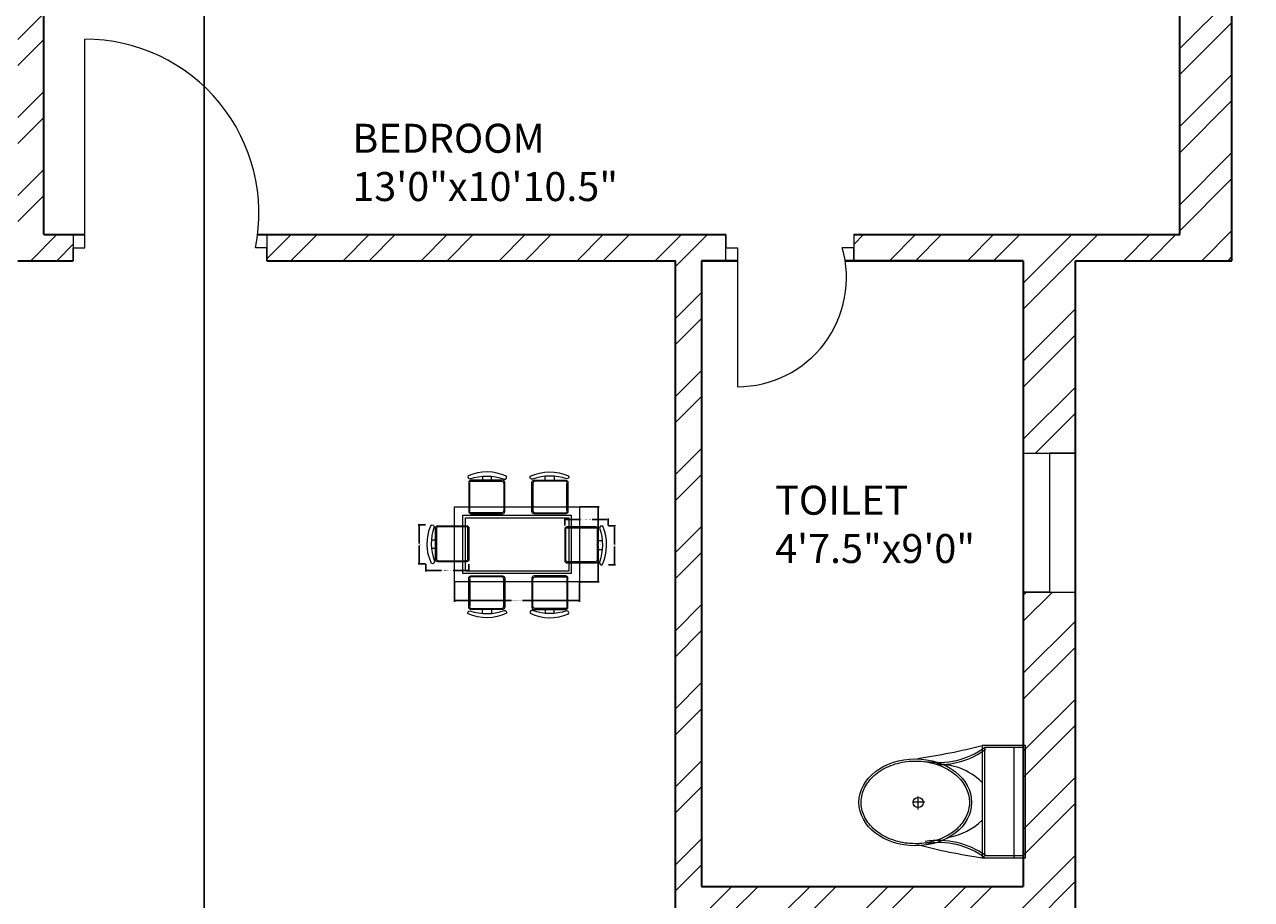
# Model space of a CAD drawing. Units: inches. Extents: x 1513 to 2170, y 1240 to 2288.
# Tile 4 of 10: x 1834 to 2045, y 1549 to 1700. Entities that reach past the tile are written whole.
import ezdxf

# ---------------------------------------------------------------- set-up
doc = ezdxf.new("R2010")
doc.units = ezdxf.units.IN
for name, color, linetype, lineweight in [('A-ANNO-DIMS', 2, 'Continuous', 18), ('A-AREA-IDEN', 7, 'Continuous', 18), ('A-DOOR', 3, 'Continuous', 18), ('A-FLOR-FIXT', 9, 'Continuous', 18), ('A-FURN', 8, 'Continuous', 18), ('A-GLAZ', 4, 'Continuous', 18), ('A-WALL', 7, 'Continuous', 35), ('A-WALL-PATT', 252, 'Continuous', 13)]:
    doc.layers.add(name, color=color, linetype=linetype, lineweight=lineweight)
doc.styles.get("Standard").update_dxf_attribs({"font": 'arial.ttf'})
doc.dimstyles.get("Standard").update_dxf_attribs({"dimtxt": 0.18, "dimasz": 0.18, "dimexe": 0.18, "dimexo": 0.0625, "dimgap": 0.09, "dimtad": 0, "dimtih": 1, "dimtoh": 1, "dimdec": 4, "dimzin": 0, "dimdsep": 46, "dimtxsty": 'Standard', "dimcen": 0.09, "dimadec": 0, "dimazin": 0, "dimtfac": 1, "dimtdec": 4, "dimtofl": 0, "dimtmove": 0, "dimatfit": 3, "dimfxl": 1, "dimtolj": 1, "dimtzin": 0, "dimarcsym": 0})

# ---------------------------------------------------------------- blocks, each defined once
blk = doc.blocks.new('A$C31115884')
for p, q in [((257.5, 466.4), (257.5, 523.2)), ((283.1, 497.7), (223.4, 497.7)), ((0, 200), (0, 0)), ((520, 200), (0, 200)), ((10, 190), (10, 10)), ((510, 190), (10, 190)), ((510, 10), (510, 190)), ((520, 0), (520, 200)), ((510, 54.5), (0, 54.5)), ((10, 10), (510, 10)), ((0, 0), (520, 0))]:
    blk.add_line(p, q)
blk.add_circle((255.6, 496.4), 23.6)
for centre, radius, start, end in [((2777.7, -204.6), 2807, 165.4549, 171.7133), ((-294.5, 403.3), 364.7, 324.2091, 9.3499), ((-294.5, 403.3), 374.7, 324.2091, 9.3499), ((805.8, 403.3), 364.7, 170.6501, 215.7909), ((3237, 905), 2807, 188.2867, 194.5451), ((139.5, 406.2), 293.5, 315.8436, 2.6563), ((805.8, 403.3), 374.7, 179.2036, 215.7909), ((383.6, 406.2), 293.5, 190.2774, 224.1564)]:
    blk.add_arc(centre, radius, start, end)
blk.add_ellipse((256.2, 509.9), major_axis=(0, -260.7), ratio=0.772727)
blk.add_open_spline([(256.2, 259.2), (263.1, 259.2), (270, 259.7), (287.8, 262.3), (298.7, 265.1), (319.9, 273.1), (330.2, 278.4), (350.1, 291.1), (359.7, 298.7), (377.7, 315.9), (386.2, 325.5), (401.7, 346.6), (408.8, 358.1), (421.3, 382.5), (426.8, 395.5), (435.9, 422.4), (439.5, 436.4), (444.8, 465.1), (446.5, 479.7), (447.9, 509.2), (447.6, 524), (445, 553.3), (442.7, 567.8), (436.3, 596), (432.1, 609.7), (421.9, 636), (416, 648.6), (402.5, 672.1), (395, 683), (378.6, 703), (369.8, 712.1), (351.1, 728), (341.3, 734.8), (320.9, 746.2), (310.4, 750.7), (288.9, 757.3), (278, 759.4), (256, 761), (245, 760.6), (223.1, 757.2), (212.3, 754.3), (191.1, 746.1), (180.8, 740.7), (160.9, 727.8), (151.4, 720.1), (133.5, 702.7), (125.1, 693), (109.6, 671.7), (102.6, 660.2), (90.2, 635.7), (84.9, 622.7), (76, 595.6), (72.4, 581.6), (67.2, 552.9), (65.6, 538.2), (64.4, 508.8), (64.8, 494), (67.5, 464.7), (69.9, 450.2), (76.6, 422), (80.8, 408.3), (91.1, 382.2), (97.2, 369.7), (110.8, 346.3), (118.4, 335.4), (134.8, 315.6), (143.7, 306.7), (162.4, 290.9), (172.3, 284.2), (192.8, 273), (203.3, 268.6), (224.8, 262.2), (235.8, 260.2), (249.9, 259.3), (253, 259.2), (256.2, 259.2)], degree=3, knots=[0, 0, 0, 0, 0.110105, 0.110105, 0.285049, 0.285049, 0.459994, 0.459994, 0.634938, 0.634938, 0.809882, 0.809882, 0.984827, 0.984827, 1.159771, 1.159771, 1.334715, 1.334715, 1.50966, 1.50966, 1.684604, 1.684604, 1.859549, 1.859549, 2.034493, 2.034493, 2.209437, 2.209437, 2.384382, 2.384382, 2.559326, 2.559326, 2.73427, 2.73427, 2.909215, 2.909215, 3.084159, 3.084159, 3.259103, 3.259103, 3.434048, 3.434048, 3.608992, 3.608992, 3.783936, 3.783936, 3.958881, 3.958881, 4.133825, 4.133825, 4.30877, 4.30877, 4.483714, 4.483714, 4.658658, 4.658658, 4.833603, 4.833603, 5.008547, 5.008547, 5.183491, 5.183491, 5.358436, 5.358436, 5.53338, 5.53338, 5.708324, 5.708324, 5.883269, 5.883269, 6.058213, 6.058213, 6.233158, 6.233158, 6.283185, 6.283185, 6.283185, 6.283185])
blk = doc.blocks.new('WIN-24')
for p, q in [((0, 24), (9, 24)), ((9, 24), (4.5, 24)), ((4.5, 24), (4.5, 0)), ((4.5, 0), (0, 0)), ((0, 0), (9, 0))]:
    blk.add_line(p, q)
blk = doc.blocks.new('TABLE-DINING')
for points in [[(0, 12.94), (21.57, 12.94), (21.57, 0), (0, 0)], [(0, 12.94), (21.57, 12.94), (21.57, 0), (0, 0)], [(1.44, 11.51), (20.13, 11.51), (20.13, 1.44), (1.44, 1.44)], [(1.44, 11.5), (20.13, 11.5), (20.13, 1.44), (1.44, 1.44)], [(1.87, 11.07), (19.7, 11.07), (19.7, 1.87), (1.87, 1.87)], [(1.87, 11.07), (19.7, 11.07), (19.7, 1.87), (1.87, 1.87)]]:
    blk.add_lwpolyline(points, close=True)
blk = doc.blocks.new('CHAIR-DINING-A')
for points in [[(0.35, 6.01, -0.175809), (6.23, 5.97, 0.578392), (6.67, 6.46, 0.214524), (0.04, 6.55, 0.552014), (0.35, 6.01, -0.065079)], [(0.35, 6.01, -0.175809), (6.23, 5.97, 0.578392), (6.67, 6.46, 0.214524), (0.04, 6.55, 0.552014), (0.35, 6.01, -0.065079)], [(4.06, 5.78), (4.06, 6.47, -0.064759)], [(4.06, 5.78), (4.06, 6.47, -0.064759)], [(5.98, 5.78), (0.53, 5.78, 0.414214), (0.14, 5.4), (0.14, 0.38, 0.414214), (0.53, 0), (5.98, 0, 0.414214), (6.36, 0.38), (6.36, 5.4, 0.414214), (5.98, 5.78)], [(5.98, 5.78), (0.53, 5.78, 0.414214), (0.14, 5.4), (0.14, 0.38, 0.414214), (0.53, 0), (5.98, 0, 0.414214), (6.36, 0.38), (6.36, 5.4, 0.414214), (5.98, 5.78)]]:
    blk.add_lwpolyline(points, format="xyb")
blk.add_lwpolyline([(2.54, 6.48), (2.54, 5.78)])
blk.add_lwpolyline([(2.54, 6.48), (2.54, 5.78)])
blk.add_lwpolyline([(0.53, 5.61), (5.81, 5.61, -0.414214), (6.19, 5.23), (6.19, 0.55, -0.414214), (5.81, 0.17), (0.53, 0.17, -0.512069), (0.32, 0.55), (0.32, 5.23, -0.512069)], format="xyb", close=True)
blk.add_lwpolyline([(0.53, 5.61), (5.81, 5.61, -0.414214), (6.19, 5.23), (6.19, 0.55, -0.414214), (5.81, 0.17), (0.53, 0.17, -0.512069), (0.32, 0.55), (0.32, 5.23, -0.512069)], format="xyb", close=True)
blk = doc.blocks.new('CHAIR-DINING-B')
for points in [[(5.98, 1.44), (0.53, 1.44, -0.414214), (0.14, 1.82), (0.14, 6.83, -0.414214), (0.53, 7.22), (5.98, 7.22, -0.414214), (6.36, 6.83), (6.36, 1.82, -0.414214), (5.98, 1.44)], [(5.98, 1.44), (0.53, 1.44, -0.414214), (0.14, 1.82), (0.14, 6.83, -0.414214), (0.53, 7.22), (5.98, 7.22, -0.414214), (6.36, 6.83), (6.36, 1.82, -0.414214), (5.98, 1.44)], [(6.23, 1.25, -0.578392), (6.67, 0.76, -0.214524), (0.04, 0.67, -0.552014), (0.35, 1.2, 0.175809), (6.23, 1.25)], [(6.23, 1.25, -0.578392), (6.67, 0.76, -0.214524), (0.04, 0.67, -0.552014), (0.35, 1.2, 0.175809), (6.23, 1.25)], [(4.06, 1.44), (4.06, 0.75, 0.064759)], [(4.06, 1.44), (4.06, 0.75, 0.064759)]]:
    blk.add_lwpolyline(points, format="xyb")
blk.add_lwpolyline([(0.53, 1.61), (5.81, 1.61, 0.414214), (6.19, 1.99), (6.19, 6.66, 0.414214), (5.81, 7.04), (0.53, 7.04, 0.512069), (0.32, 6.66), (0.32, 1.99, 0.512069)], format="xyb", close=True)
blk.add_lwpolyline([(0.53, 1.61), (5.81, 1.61, 0.414214), (6.19, 1.99), (6.19, 6.66, 0.414214), (5.81, 7.04), (0.53, 7.04, 0.512069), (0.32, 6.66), (0.32, 1.99, 0.512069)], format="xyb", close=True)
blk.add_lwpolyline([(2.54, 0.74), (2.54, 1.44)])
blk.add_lwpolyline([(2.54, 0.74), (2.54, 1.44)])
blk = doc.blocks.new('*D17')
at = {"layer": 'A-ANNO-DIMS', "color": 0, "lineweight": -2, "transparency": 16777216}
for p, q in [((1926.73, 1613.76), (1926.73, 1615)), ((1926.91, 1614.82), (1929.47, 1614.82)), ((1934.02, 1614.82), (1931.47, 1614.82)), ((1934.2, 1613.76), (1934.2, 1615))]:
    blk.add_line(p, q, dxfattribs=at)
at = {"layer": 'A-ANNO-DIMS', "color": 0, "transparency": 16777216}
for points in [[(1926.91, 1614.85), (1926.91, 1614.79), (1926.73, 1614.82)], [(1934.02, 1614.85), (1934.02, 1614.79), (1934.2, 1614.82)]]:
    blk.add_solid(points, dxfattribs=at)
at = {"layer": 'Defpoints', "color": 0, "transparency": 16777216}
for p in [(1926.73, 1613.7), (1934.2, 1614.82), (1934.2, 1613.7)]:
    blk.add_point(p, dxfattribs=at)
at = {"layer": 'A-ANNO-DIMS', "color": 0, "transparency": 16777216, "insert": (1930.47, 1614.82), "char_height": 0.18, "attachment_point": 5}
blk.add_mtext('\\A1;CHAIR A 7 TYP.', dxfattribs=at)
blk = doc.blocks.new('*D18')
at = {"layer": 'A-ANNO-DIMS', "color": 0, "lineweight": -2, "transparency": 16777216}
for p, q in [((1934.26, 1613.7), (1935.5, 1613.7)), ((1935.32, 1613.52), (1935.32, 1610.51)), ((1935.32, 1607.15), (1935.32, 1610.15)), ((1934.26, 1606.97), (1935.5, 1606.97))]:
    blk.add_line(p, q, dxfattribs=at)
at = {"layer": 'A-ANNO-DIMS', "color": 0, "transparency": 16777216}
for points in [[(1935.29, 1613.52), (1935.35, 1613.52), (1935.32, 1613.7)], [(1935.29, 1607.15), (1935.35, 1607.15), (1935.32, 1606.97)]]:
    blk.add_solid(points, dxfattribs=at)
at = {"layer": 'Defpoints', "color": 0, "transparency": 16777216}
for p in [(1934.2, 1613.7), (1934.2, 1606.97), (1935.32, 1606.97)]:
    blk.add_point(p, dxfattribs=at)
at = {"layer": 'A-ANNO-DIMS', "color": 0, "transparency": 16777216, "insert": (1935.32, 1610.33), "char_height": 0.18, "attachment_point": 5}
blk.add_mtext('\\A1;7 TYP.', dxfattribs=at)
blk = doc.blocks.new('*D19')
at = {"layer": 'A-ANNO-DIMS', "color": 0, "lineweight": -2, "transparency": 16777216}
for p, q in [((1902.74, 1607.09), (1902.74, 1605.85)), ((1910.21, 1607.09), (1910.21, 1605.85)), ((1902.92, 1606.03), (1905.47, 1606.03)), ((1910.03, 1606.03), (1907.47, 1606.03))]:
    blk.add_line(p, q, dxfattribs=at)
at = {"layer": 'A-ANNO-DIMS', "color": 0, "transparency": 16777216}
for points in [[(1902.92, 1606.06), (1902.92, 1606), (1902.74, 1606.03)], [(1910.03, 1606.06), (1910.03, 1606), (1910.21, 1606.03)]]:
    blk.add_solid(points, dxfattribs=at)
at = {"layer": 'Defpoints', "color": 0, "transparency": 16777216}
for p in [(1902.74, 1607.15), (1910.21, 1607.15), (1910.21, 1606.03)]:
    blk.add_point(p, dxfattribs=at)
at = {"layer": 'A-ANNO-DIMS', "color": 0, "transparency": 16777216, "insert": (1906.47, 1606.03), "char_height": 0.18, "attachment_point": 5}
blk.add_mtext('\\A1;CHAIR B 7 TYP.', dxfattribs=at)
blk = doc.blocks.new('*D20')
at = {"layer": 'A-ANNO-DIMS', "color": 0, "lineweight": -2, "transparency": 16777216}
for p, q in [((1902.68, 1613.89), (1901.44, 1613.89)), ((1901.62, 1613.71), (1901.62, 1610.7)), ((1901.62, 1607.33), (1901.62, 1610.34)), ((1902.68, 1607.15), (1901.44, 1607.15))]:
    blk.add_line(p, q, dxfattribs=at)
at = {"layer": 'A-ANNO-DIMS', "color": 0, "transparency": 16777216}
for points in [[(1901.59, 1613.71), (1901.65, 1613.71), (1901.62, 1613.89)], [(1901.59, 1607.33), (1901.65, 1607.33), (1901.62, 1607.15)]]:
    blk.add_solid(points, dxfattribs=at)
at = {"layer": 'Defpoints', "color": 0, "transparency": 16777216}
for p in [(1902.74, 1613.89), (1901.62, 1607.15), (1902.74, 1607.15)]:
    blk.add_point(p, dxfattribs=at)
at = {"layer": 'A-ANNO-DIMS', "color": 0, "transparency": 16777216, "insert": (1901.62, 1610.52), "char_height": 0.18, "attachment_point": 5}
blk.add_mtext('\\A1;7 TYP.', dxfattribs=at)
blk = doc.blocks.new('*D21')
at = {"layer": 'A-ANNO-DIMS', "color": 0, "lineweight": -2, "transparency": 16777216}
for p, q in [((1907.71, 1603.98), (1907.71, 1600.63)), ((1929.28, 1603.98), (1929.28, 1600.63)), ((1907.89, 1600.81), (1917.53, 1600.81)), ((1929.1, 1600.81), (1919.46, 1600.81))]:
    blk.add_line(p, q, dxfattribs=at)
at = {"layer": 'A-ANNO-DIMS', "color": 0, "transparency": 16777216}
for points in [[(1907.89, 1600.84), (1907.89, 1600.78), (1907.71, 1600.81)], [(1929.1, 1600.84), (1929.1, 1600.78), (1929.28, 1600.81)]]:
    blk.add_solid(points, dxfattribs=at)
at = {"layer": 'Defpoints', "color": 0, "transparency": 16777216}
for p in [(1907.71, 1604.04), (1929.28, 1604.04), (1929.28, 1600.81)]:
    blk.add_point(p, dxfattribs=at)
at = {"layer": 'A-ANNO-DIMS', "color": 0, "transparency": 16777216, "insert": (1918.5, 1600.81), "char_height": 0.18, "attachment_point": 5}
blk.add_mtext('\\A1;TABLE 22 TYP.', dxfattribs=at)
blk = doc.blocks.new('*D22')
at = {"layer": 'A-ANNO-DIMS', "color": 0, "lineweight": -2, "transparency": 16777216}
for p, q in [((1929.35, 1616.99), (1932.7, 1616.99)), ((1932.52, 1616.81), (1932.52, 1610.7)), ((1932.52, 1604.22), (1932.52, 1610.33)), ((1929.35, 1604.04), (1932.7, 1604.04))]:
    blk.add_line(p, q, dxfattribs=at)
at = {"layer": 'A-ANNO-DIMS', "color": 0, "transparency": 16777216}
for points in [[(1932.49, 1616.81), (1932.55, 1616.81), (1932.52, 1616.99)], [(1932.49, 1604.22), (1932.55, 1604.22), (1932.52, 1604.04)]]:
    blk.add_solid(points, dxfattribs=at)
at = {"layer": 'Defpoints', "color": 0, "transparency": 16777216}
for p in [(1929.28, 1616.99), (1932.52, 1616.99), (1929.28, 1604.04)]:
    blk.add_point(p, dxfattribs=at)
at = {"layer": 'A-ANNO-DIMS', "color": 0, "transparency": 16777216, "insert": (1932.52, 1610.52), "char_height": 0.18, "attachment_point": 5}
blk.add_mtext('\\A1;13 TYP.', dxfattribs=at)
blk = doc.blocks.new('*D26')
at = {"layer": 'A-ANNO-DIMS', "color": 0, "lineweight": -2, "transparency": 16777216}
for p, q in [((2014.91, 2214.48), (2087.18, 2214.48)), ((2087, 2214.3), (2087, 1802.16)), ((2087, 1389.66), (2087, 1801.8)), ((1937.43, 1389.48), (2087.18, 1389.48))]:
    blk.add_line(p, q, dxfattribs=at)
at = {"layer": 'A-ANNO-DIMS', "color": 0, "transparency": 16777216}
for points in [[(2086.97, 2214.3), (2087.03, 2214.3), (2087, 2214.48)], [(2086.97, 1389.66), (2087.03, 1389.66), (2087, 1389.48)]]:
    blk.add_solid(points, dxfattribs=at)
at = {"layer": 'Defpoints', "color": 0, "transparency": 16777216}
for p in [(2014.85, 2214.48), (2087, 2214.48), (1937.37, 1389.48)]:
    blk.add_point(p, dxfattribs=at)
at = {"layer": 'A-ANNO-DIMS', "color": 0, "transparency": 16777216, "insert": (2087, 1801.98), "char_height": 0.18, "attachment_point": 5}
blk.add_mtext('\\A1;825', dxfattribs=at)
blk = doc.blocks.new('*D36')
at = {"layer": 'A-ANNO-DIMS', "color": 0, "lineweight": -2, "transparency": 16777216}
for p, q in [((1829.49, 1887.42), (1829.49, 1344.15)), ((1864.51, 1887.42), (1864.51, 1344.15)), ((1829.67, 1344.33), (1846.61, 1344.33)), ((1864.33, 1344.33), (1847.39, 1344.33))]:
    blk.add_line(p, q, dxfattribs=at)
at = {"layer": 'A-ANNO-DIMS', "color": 0, "transparency": 16777216}
for points in [[(1829.67, 1344.36), (1829.67, 1344.3), (1829.49, 1344.33)], [(1864.33, 1344.36), (1864.33, 1344.3), (1864.51, 1344.33)]]:
    blk.add_solid(points, dxfattribs=at)
at = {"layer": 'Defpoints', "color": 0, "transparency": 16777216}
for p in [(1829.49, 1887.48), (1864.51, 1887.48), (1864.51, 1344.33)]:
    blk.add_point(p, dxfattribs=at)
at = {"layer": 'A-ANNO-DIMS', "color": 0, "transparency": 16777216, "insert": (1847, 1344.33), "char_height": 0.18, "attachment_point": 5}
blk.add_mtext('\\A1;35.02', dxfattribs=at)

msp = doc.modelspace()

# ---------------------------------------------------------------- hatches: boundary and pattern name
at = {"layer": 'A-WALL-PATT'}
h = msp.add_hatch(dxfattribs=at)
h.set_pattern_fill('ANSI32', color=256)
h.paths.add_polyline_path([(2041.852, 1719.48), (2014.852, 1719.48), (2014.852, 1734.444), (2005.852, 1734.444), (2005.852, 1710.48), (2032.852, 1710.48), (2032.852, 1663.98), (1976.619, 1663.98), (1976.619, 1659.48), (2005.852, 1659.48), (2005.852, 1626.27), (2014.852, 1626.27), (2014.852, 1659.48), (2041.852, 1659.48)])
h.paths.add_polyline_path([(1954.521, 1663.98), (1875.357, 1663.98), (1875.357, 1659.48), (1945.852, 1659.48), (1945.852, 1546.98), (1950.352, 1546.98), (2005.852, 1546.98), (2005.852, 1422.48), (1985.47, 1422.48), (1985.47, 1413.48), (2014.852, 1413.48), (2014.852, 1602.27), (2005.852, 1602.27), (2005.852, 1551.48), (1950.352, 1551.48), (1950.352, 1659.48), (1954.521, 1659.48)])
h.paths.add_polyline_path([(1949.47, 1422.48), (1937.366, 1422.48), (1937.366, 1413.48), (1949.47, 1413.48)], flags=0)
h.paths.add_polyline_path([(1937.366, 1422.48), (1908.866, 1422.48), (1908.866, 1546.98), (1805.486, 1546.98), (1805.486, 1542.48), (1904.366, 1542.48), (1904.366, 1451.2), (1897.222, 1451.2), (1897.222, 1442.2), (1904.366, 1442.2), (1904.366, 1422.48), (1904.366, 1413.48), (1904.366, 1389.48), (1908.866, 1389.48), (1908.866, 1413.48), (1932.866, 1413.48), (1932.866, 1389.48), (1937.366, 1389.48)])
h.paths.add_polyline_path([(1830.254, 1442.2), (1844.144, 1442.2), (1844.144, 1451.2), (1830.254, 1451.2), (1821.254, 1451.2), (1821.254, 1422.48), (1766.366, 1422.48), (1766.366, 1542.48), (1770.265, 1542.48), (1770.265, 1546.98), (1758.774, 1546.98), (1758.774, 1544.73), (1758.774, 1542.48), (1761.866, 1542.48), (1761.866, 1389.48), (1779.454, 1389.48), (1779.454, 1398.48), (1770.866, 1398.48), (1770.866, 1413.48), (1830.254, 1413.48)])
h.paths.add_polyline_path([(1686.156, 1451.2), (1677.156, 1451.2), (1677.156, 1422.48), (1623.866, 1422.48), (1623.866, 1460.073), (1614.866, 1460.073), (1614.866, 1413.48), (1686.156, 1413.48)])
h.paths.add_polyline_path([(1761.866, 1422.48), (1686.156, 1422.48), (1686.156, 1413.48), (1761.866, 1413.48)])
h.paths.add_polyline_path([(1623.866, 1542.48), (1688.266, 1542.48), (1688.266, 1544.73), (1688.266, 1546.98), (1623.866, 1546.98), (1623.866, 1560.442), (1614.866, 1560.442), (1614.866, 1520.073), (1619.366, 1520.073), (1623.866, 1520.073)])
h.paths.add_polyline_path([(1623.866, 1600.98), (1715.366, 1600.98), (1715.366, 1546.98), (1711.055, 1546.98), (1711.055, 1542.48), (1719.866, 1542.48), (1726.867, 1542.48), (1726.867, 1544.73), (1726.867, 1546.98), (1719.866, 1546.98), (1719.866, 1600.98), (1719.866, 1608.301), (1717.616, 1608.301), (1715.366, 1608.301), (1715.366, 1605.48), (1623.866, 1605.48), (1623.866, 1620.254), (1614.866, 1620.254), (1614.866, 1584.442), (1623.866, 1584.442)])
h.paths.add_polyline_path([(1623.866, 1659.48), (1715.366, 1659.48), (1715.366, 1629.2), (1719.866, 1629.2), (1719.866, 1659.48), (1767.866, 1659.48), (1767.866, 1629.2), (1772.366, 1629.2), (1772.366, 1663.98), (1578.866, 1663.98), (1578.866, 1661.73), (1578.866, 1659.48), (1578.866, 1635.48), (1583.366, 1635.48), (1583.366, 1654.98), (1614.866, 1654.98), (1614.866, 1644.254), (1619.366, 1644.254), (1623.866, 1644.254)])
h.paths.add_polyline_path([(1788.587, 1798.98), (1788.587, 1803.48), (1623.866, 1803.48), (1623.866, 1887.48), (1829.49, 1887.48), (1829.49, 1891.98), (1829.49, 1896.48), (1748.366, 1896.48), (1743.866, 1896.48), (1623.866, 1896.48), (1623.866, 1904.333), (1619.366, 1904.333), (1614.866, 1904.333), (1614.866, 1896.48), (1578.866, 1896.48), (1578.866, 1887.48), (1614.866, 1887.48), (1614.866, 1803.48), (1578.866, 1803.48), (1578.866, 1794.48), (1626.866, 1794.48), (1788.587, 1794.48)])
h.paths.add_polyline_path([(1635.866, 1794.48), (1626.866, 1794.48), (1626.866, 1763.627), (1631.366, 1763.627), (1635.866, 1763.627)])
h.paths.add_polyline_path([(1635.866, 1703.627), (1626.866, 1703.627), (1626.866, 1663.98), (1635.866, 1663.98)])
h.paths.add_polyline_path([(1587.866, 2016.48), (1614.866, 2016.48), (1623.866, 2016.48), (1707.767, 2016.48), (1707.767, 2018.73), (1707.767, 2020.98), (1706.366, 2020.98), (1706.366, 2025.944), (1701.866, 2025.944), (1701.866, 2020.98), (1623.866, 2020.98), (1623.866, 2045.903), (1614.866, 2045.903), (1614.866, 2025.48), (1583.366, 2025.48), (1583.366, 2040.48), (1578.866, 2040.48), (1578.866, 2016.48), (1578.866, 1956.48), (1614.866, 1956.48), (1614.866, 1946.333), (1623.866, 1946.333), (1623.866, 1965.48), (1587.866, 1965.48)])
h.paths.add_polyline_path([(1748.366, 2016.48), (1748.366, 2025.48), (1743.866, 2025.48), (1739.366, 2025.48), (1739.366, 2020.98), (1738.09, 2020.98), (1738.09, 2016.48), (1743.866, 2016.48), (1743.866, 1896.48), (1748.366, 1896.48)])
h.paths.add_polyline_path([(1746.736, 2085.48), (1623.866, 2085.48), (1623.866, 2205.48), (1657.136, 2205.48), (1657.136, 2214.48), (1614.866, 2214.48), (1614.866, 2069.903), (1623.866, 2069.903), (1623.866, 2080.98), (1683.866, 2080.98), (1701.866, 2080.98), (1701.866, 2046.743), (1706.366, 2046.743), (1706.366, 2080.98), (1746.736, 2080.98)])
h = msp.add_hatch(dxfattribs=at)
h.set_pattern_fill('ANSI32', color=256)
h.paths.add_polyline_path([(1744.852, 2209.98), (1762.042, 2209.98), (1762.042, 2214.48), (1715.345, 2214.48), (1715.345, 2205.48), (1735.852, 2205.48), (1735.852, 2161.98), (1733.253, 2161.98), (1719.866, 2161.98), (1719.866, 2112.429), (1724.366, 2112.429), (1724.366, 2152.98), (1762.042, 2152.98), (1870.852, 2152.98), (1870.852, 2080.98), (1875.352, 2080.98), (1878.245, 2080.98), (1878.245, 2083.23), (1878.245, 2085.48), (1875.352, 2085.48), (1875.352, 2173.929), (1881.628, 2173.929), (1881.628, 2178.429), (1881.628, 2182.929), (1875.352, 2182.929), (1875.352, 2214.48), (1858.335, 2214.48), (1858.335, 2209.98), (1866.352, 2209.98), (1866.352, 2161.98), (1762.042, 2161.98), (1744.852, 2161.98)])
h.paths.add_polyline_path([(2014.852, 2214.48), (1944.011, 2214.48), (1944.011, 2182.929), (1938.347, 2182.929), (1938.347, 2173.929), (1953.011, 2173.929), (1953.011, 2182.929), (1953.011, 2205.48), (2005.852, 2205.48), (2005.852, 2085.48), (1955.061, 2085.48), (1955.061, 2080.98), (2005.852, 2080.98), (2005.852, 2068.903), (2014.852, 2068.903)])
h.paths.add_polyline_path([(2014.852, 2044.903), (2005.852, 2044.903), (2005.852, 2020.98), (1926.352, 2020.98), (1926.352, 2080.98), (1930.882, 2080.98), (1930.882, 2083.23), (1930.882, 2085.48), (1921.852, 2085.48), (1915.536, 2085.48), (1915.536, 2083.23), (1915.536, 2080.98), (1921.852, 2080.98), (1921.852, 2020.98), (1916.378, 2020.98), (1916.378, 2018.73), (1916.378, 2016.48), (2005.852, 2016.48), (2005.852, 2009.442), (2014.852, 2009.442), (2014.852, 2016.48), (2029.852, 2016.48), (2041.852, 2016.48), (2041.852, 2040.48), (2037.352, 2040.48), (2037.352, 2036.595), (2037.352, 2020.98), (2014.852, 2020.98)])
h.paths.add_polyline_path([(2041.852, 1956.48), (2014.852, 1956.48), (2014.852, 1963.797), (2005.852, 1963.797), (2005.852, 1947.48), (2032.852, 1947.48), (2032.852, 1896.48), (1978.852, 1896.48), (1978.852, 1891.98), (1978.852, 1887.48), (2005.852, 1887.48), (2005.852, 1862.401), (2014.852, 1862.401), (2014.852, 1887.48), (2037.352, 1887.48), (2037.352, 1863.48), (2041.852, 1863.48), (2041.852, 1887.48), (2041.852, 1896.48)], flags=17)
h.paths.add_polyline_path([(1885.852, 1896.48), (1885.852, 1920.48), (1878.866, 1920.48), (1878.866, 2016.48), (1881.925, 2016.48), (1881.925, 2018.73), (1881.925, 2020.98), (1874.366, 2020.98), (1874.366, 1896.48), (1864.508, 1896.48), (1864.508, 1887.48), (1876.852, 1887.48), (1876.852, 1855.773), (1885.852, 1855.773), (1885.852, 1868.947), (1942.852, 1868.947), (1942.852, 1803.48), (1885.852, 1803.48), (1885.852, 1817.861), (1876.852, 1817.861), (1876.852, 1803.48), (1825.976, 1803.48), (1825.976, 1798.98), (1825.976, 1794.48), (1832.366, 1794.48), (1832.366, 1663.98), (1832.366, 1659.48), (1841.939, 1659.48), (1841.939, 1661.73), (1841.939, 1663.98), (1836.866, 1663.98), (1836.866, 1794.48), (1992.866, 1794.48), (2005.852, 1794.48), (2005.852, 1784.304), (2010.352, 1784.304), (2014.852, 1784.304), (2014.852, 1794.48), (2041.852, 1794.48), (2041.852, 1803.48), (2014.852, 1803.48), (2014.852, 1838.401), (2005.852, 1838.401), (2005.852, 1803.48), (1951.852, 1803.48), (1951.852, 1887.48), (1956.114, 1887.48), (1956.114, 1891.98), (1956.114, 1896.48), (1951.852, 1896.48), (1951.852, 1920.48), (1947.352, 1920.48), (1947.352, 1896.48), (1942.852, 1896.48), (1942.852, 1877.947), (1885.852, 1877.947)])

# ---------------------------------------------------------------- linework, layer by layer
at = {"layer": 'A-DOOR'}
for p, q in [((1843.939, 1661.73), (1843.939, 1697.73)), ((1841.939, 1663.98), (1841.939, 1659.48)), ((1875.357, 1663.98), (1875.357, 1659.48)), ((1954.521, 1659.48), (1954.521, 1663.98)), ((1954.521, 1663.98), (1954.521, 1661.73)), ((1976.619, 1663.98), (1976.619, 1659.48)), ((1841.939, 1659.48), (1841.939, 1661.73)), ((1841.939, 1661.73), (1843.939, 1661.73)), ((1875.357, 1661.73), (1873.357, 1661.73)), ((1875.357, 1659.48), (1875.357, 1661.73)), ((1954.521, 1661.73), (1956.521, 1661.73)), ((1956.521, 1661.73), (1956.521, 1637.73)), ((1976.619, 1661.73), (1974.619, 1661.73)), ((1976.619, 1659.48), (1976.619, 1661.73))]:
    msp.add_line(p, q, dxfattribs=at)
for centre, radius, start, end in [((1843.939, 1667.71), 30.02, 348.50896, 90), ((1956.521, 1656.553), 18.823, 270, 15.96234)]:
    msp.add_arc(centre, radius, start, end, dxfattribs=at)
at = {"layer": 'A-FURN'}
for points in [[(1910.382, 1621.827, -0.1758092), (1916.257, 1621.783, 0.5783921), (1916.702, 1622.272, 0.2145244), (1910.071, 1622.361, 0.552014), (1910.382, 1621.827, -0.065079)], [(1910.382, 1621.827, -0.1758092), (1916.257, 1621.783, 0.5783921), (1916.702, 1622.272, 0.2145244), (1910.071, 1622.361, 0.552014), (1910.382, 1621.827, -0.065079)], [(1914.092, 1621.592), (1914.092, 1622.281, -0.0647586)], [(1914.092, 1621.591), (1914.092, 1622.281, -0.0647586)], [(1916.007, 1621.592), (1910.554, 1621.592, 0.4142136), (1910.172, 1621.21), (1910.172, 1616.195, 0.4142136), (1910.554, 1615.814), (1916.007, 1615.814, 0.4142136), (1916.389, 1616.195), (1916.389, 1621.21, 0.4142136), (1916.007, 1621.592)], [(1916.007, 1621.591), (1910.554, 1621.591, 0.4142136), (1910.172, 1621.21), (1910.172, 1616.195, 0.4142136), (1910.554, 1615.814), (1916.007, 1615.814, 0.4142136), (1916.389, 1616.195), (1916.389, 1621.21, 0.4142136), (1916.007, 1621.591)], [(1916.007, 1599.3), (1910.554, 1599.3, -0.4142136), (1910.172, 1599.682), (1910.172, 1604.696, -0.4142136), (1910.554, 1605.078), (1916.007, 1605.078, -0.4142136), (1916.389, 1604.696), (1916.389, 1599.682, -0.4142136), (1916.007, 1599.3)], [(1916.007, 1599.3), (1910.554, 1599.3, -0.4142136), (1910.172, 1599.682), (1910.172, 1604.696, -0.4142136), (1910.554, 1605.078), (1916.007, 1605.078, -0.4142136), (1916.389, 1604.696), (1916.389, 1599.682, -0.4142136), (1916.007, 1599.3)], [(1926.905, 1599.3, 0.4142136), (1927.287, 1599.682), (1927.287, 1604.696, 0.4142136), (1926.905, 1605.078), (1921.452, 1605.078, 0.4142136), (1921.07, 1604.696), (1921.07, 1599.682, 0.4142136), (1921.452, 1599.3), (1926.905, 1599.3)], [(1926.905, 1599.3, 0.4142136), (1927.287, 1599.682), (1927.287, 1604.696, 0.4142136), (1926.905, 1605.078), (1921.452, 1605.078, 0.4142136), (1921.07, 1604.696), (1921.07, 1599.682, 0.4142136), (1921.452, 1599.3), (1926.905, 1599.3)], [(1916.257, 1599.109, -0.5783921), (1916.702, 1598.62, -0.2145244), (1910.071, 1598.531, -0.552014), (1910.382, 1599.064, 0.1758093), (1916.257, 1599.109)], [(1916.257, 1599.109, -0.5783921), (1916.702, 1598.619, -0.2145244), (1910.071, 1598.53, -0.552014), (1910.382, 1599.064, 0.1758093), (1916.257, 1599.109)], [(1914.092, 1599.3), (1914.092, 1598.611, 0.0647586)], [(1914.092, 1599.3), (1914.092, 1598.61, 0.0647586)], [(1927.077, 1599.064, -0.1758093), (1921.202, 1599.109, 0.5783921), (1920.757, 1598.62, 0.2145244), (1927.388, 1598.531, 0.552014), (1927.077, 1599.064, -0.065079)], [(1927.077, 1599.064, -0.1758093), (1921.202, 1599.109, 0.5783921), (1920.757, 1598.619, 0.2145244), (1927.388, 1598.53, 0.552014), (1927.077, 1599.064, -0.065079)], [(1923.367, 1599.3), (1923.367, 1598.611, -0.0647586)], [(1923.367, 1599.3), (1923.367, 1598.61, -0.0647586)]]:
    msp.add_lwpolyline(points, format="xyb", dxfattribs=at)
for points in [[(1912.565, 1622.294), (1912.565, 1621.592)], [(1912.565, 1622.294), (1912.565, 1621.591)], [(1912.565, 1598.598), (1912.565, 1599.3)], [(1912.565, 1598.598), (1912.565, 1599.3)], [(1924.894, 1598.598), (1924.894, 1599.3)], [(1924.894, 1598.598), (1924.894, 1599.3)]]:
    msp.add_lwpolyline(points, dxfattribs=at)
for points in [[(1910.556, 1621.42), (1915.836, 1621.42, -0.4142136), (1916.217, 1621.038), (1916.217, 1616.367, -0.4142136), (1915.836, 1615.986), (1910.556, 1615.986, -0.5120695), (1910.344, 1616.367), (1910.344, 1621.038, -0.5120695)], [(1910.556, 1621.419), (1915.836, 1621.419, -0.4142136), (1916.217, 1621.038), (1916.217, 1616.367, -0.4142136), (1915.836, 1615.985), (1910.556, 1615.985, -0.5120695), (1910.344, 1616.367), (1910.344, 1621.038, -0.5120695)], [(1910.556, 1599.472), (1915.836, 1599.472, 0.4142136), (1916.217, 1599.854), (1916.217, 1604.525, 0.4142136), (1915.836, 1604.906), (1910.556, 1604.906, 0.5120695), (1910.344, 1604.525), (1910.344, 1599.854, 0.5120695)], [(1910.556, 1599.472), (1915.836, 1599.472, 0.4142136), (1916.217, 1599.853), (1916.217, 1604.524, 0.4142136), (1915.836, 1604.906), (1910.556, 1604.906, 0.5120695), (1910.344, 1604.524), (1910.344, 1599.853, 0.5120695)], [(1926.903, 1599.472), (1921.623, 1599.472, -0.4142136), (1921.242, 1599.854), (1921.242, 1604.525, -0.4142136), (1921.623, 1604.906), (1926.903, 1604.906, -0.5120695), (1927.115, 1604.525), (1927.115, 1599.854, -0.5120695)], [(1926.903, 1599.472), (1921.623, 1599.472, -0.4142136), (1921.242, 1599.853), (1921.242, 1604.524, -0.4142136), (1921.623, 1604.906), (1926.903, 1604.906, -0.5120695), (1927.115, 1604.524), (1927.115, 1599.853, -0.5120695)]]:
    msp.add_lwpolyline(points, format="xyb", close=True, dxfattribs=at)
at = {"layer": 'A-WALL'}
for p, q in [((1836.866, 1663.98), (1836.866, 1794.48)), ((2041.852, 1659.48), (2041.852, 1719.48)), ((2032.852, 1663.98), (2032.852, 1710.48)), ((1836.866, 1663.98), (1843.939, 1663.98)), ((1873.726, 1663.98), (1954.521, 1663.98)), ((1976.619, 1663.98), (2032.852, 1663.98)), ((1832.366, 1659.48), (1841.939, 1659.48)), ((1875.357, 1659.48), (1945.852, 1659.48)), ((1945.852, 1546.98), (1945.852, 1659.48)), ((1950.352, 1659.48), (1950.352, 1551.48)), ((1950.352, 1659.48), (1956.521, 1659.48)), ((1956.521, 1659.48), (1950.352, 1659.48)), ((2005.852, 1659.48), (1975.115, 1659.48)), ((1975.115, 1659.48), (2005.852, 1659.48)), ((2005.852, 1659.48), (2005.852, 1551.48)), ((2014.852, 1413.48), (2014.852, 1659.48)), ((2014.852, 1659.48), (2041.852, 1659.48)), ((1950.352, 1551.48), (2005.852, 1551.48))]:
    msp.add_line(p, q, dxfattribs=at)

# ---------------------------------------------------------------- block references
at = {"layer": 'A-FLOR-FIXT', "xscale": 0.0372717239612423, "yscale": 0.0372717239612423, "zscale": 0.0372717239612423, "rotation": 89.99999999999999}
msp.add_blockref('A$C31115884', (2006.225, 1556.439), dxfattribs=at)
at = {"layer": 'A-FURN'}
for name, p, rotation in [('CHAIR-DINING-B', (1927.432, 1623.029), 180), ('CHAIR-DINING-B', (1902.99, 1613.871), 270), ('CHAIR-DINING-A', (1926.733, 1613.684), 270)]:
    msp.add_blockref(name, p, dxfattribs=dict(at, rotation=rotation))
msp.add_blockref('TABLE-DINING', (1907.717, 1604.043), dxfattribs=at)
at = {"layer": 'A-GLAZ'}
msp.add_blockref('WIN-24', (2005.85, 1602.27), dxfattribs=at)

# ---------------------------------------------------------------- texts
at = {"layer": 'A-AREA-IDEN', "char_height": 5, "attachment_point": 1}
for s, width, insert in [('BEDROOM\\P13\'0"x10\'10.5"', 166.79693, (1890.089, 1683.118)), ('TOILET\\P4\'7.5"x9\'0"', 111.60147, (1963.044, 1620.641))]:
    msp.add_mtext_dynamic_manual_height_columns(s, width=width, gutter_width=12.5, heights=[0], dxfattribs=dict(at, insert=insert))

# ---------------------------------------------------------------- dimensions: what is measured, and where the dimension line sits
at = {"layer": 'A-ANNO-DIMS'}
dim = msp.add_linear_dim(base=(2087.002, 2214.48), p1=(1937.366, 1389.48), p2=(2014.852, 2214.48), angle=90, dimstyle='Standard', override={"dimdec": 0, "dimlfac": 1, "dimrnd": 0, "dimzin": 0, "dimdsep": 46, "dimlunit": 2}, dxfattribs=at)
dim.commit()
dim.dimension.update_dxf_attribs({"geometry": '*D26', "text_midpoint": (2087.002, 1801.98)})
dim = msp.add_linear_dim(base=(1864.508, 1344.33), p1=(1829.49, 1887.48), p2=(1864.508, 1887.48), dimstyle='Standard', override={"dimdec": 2, "dimlfac": 1, "dimrnd": 0, "dimzin": 0, "dimdsep": 46, "dimlunit": 2}, dxfattribs=at)
dim.commit()
dim.dimension.update_dxf_attribs({"geometry": '*D36', "text_midpoint": (1846.999, 1344.33)})
for base, p1, p2, text, picture, middle in [((1934.201, 1614.819), (1926.734, 1613.698), (1934.201, 1613.698), 'CHAIR A <> TYP.', '*D17', (1930.468, 1614.819)), ((1910.205, 1606.034), (1902.738, 1607.154), (1910.205, 1607.154), 'CHAIR B <> TYP.', '*D19', (1906.471, 1606.034)), ((1929.283, 1600.809), (1907.714, 1604.044), (1929.283, 1604.044), 'TABLE <> TYP.', '*D21', (1918.498, 1600.809))]:
    dim = msp.add_linear_dim(base=base, p1=p1, p2=p2, text=text, dimstyle='Standard', override={"dimdec": 0, "dimlfac": 1, "dimrnd": 0, "dimzin": 0, "dimdsep": 46, "dimlunit": 2}, dxfattribs=at)
    dim.commit()
    dim.dimension.update_dxf_attribs({"geometry": picture, "text_midpoint": middle})
for base, p1, p2, angle, picture, middle in [((1932.518, 1616.986), (1929.283, 1604.044), (1929.283, 1616.986), 90, '*D22', (1932.518, 1610.515)), ((1901.617, 1607.154), (1902.738, 1613.885), (1902.738, 1607.154), 270, '*D20', (1901.617, 1610.52)), ((1935.322, 1606.967), (1934.201, 1613.698), (1934.201, 1606.967), 270, '*D18', (1935.322, 1610.333))]:
    dim = msp.add_linear_dim(base=base, p1=p1, p2=p2, angle=angle, text='<> TYP.', dimstyle='Standard', override={"dimdec": 0, "dimlfac": 1, "dimrnd": 0, "dimzin": 0, "dimdsep": 46, "dimlunit": 2}, dxfattribs=at)
    dim.commit()
    dim.dimension.update_dxf_attribs({"geometry": picture, "text_midpoint": middle})

doc.saveas('drawing.dxf')
